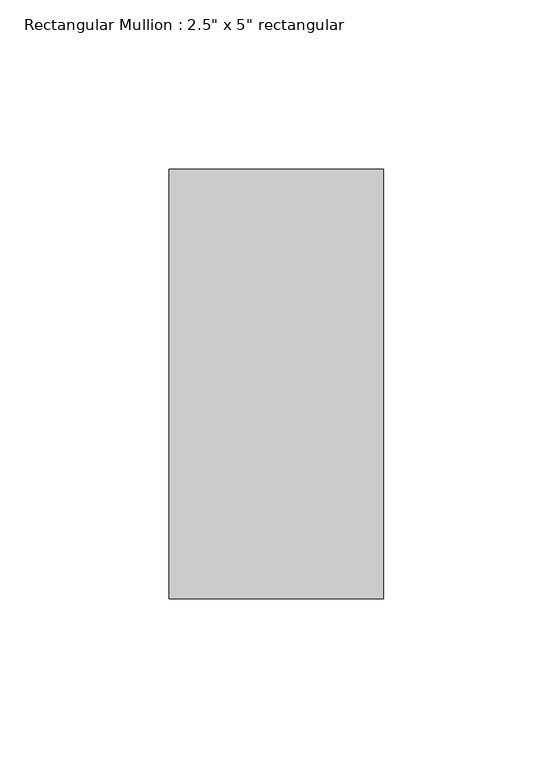
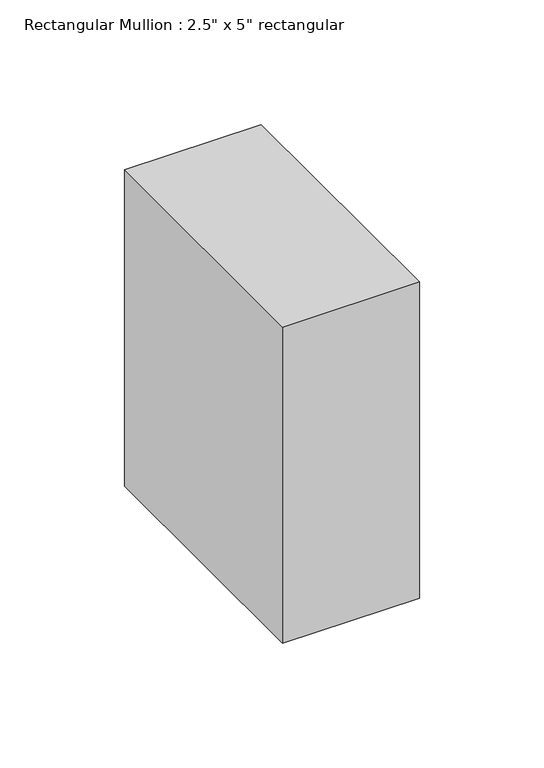
"""IFC4 building model written with IfcOpenShell, lengths in millimetres: member geometry."""

from ifc_helpers import new_model, si_unit, frame, origin, place, context, project, spatial, polyline, outline, extrude, source, transform, mapped, element, save


def member_6ed1261f(model_context):
    return source(origin(), model_context, "Body", "SweptSolid", [
        extrude(outline(polyline([(0.0, 63.5), (0.0, -63.5), (-63.5, -63.5), (-63.5, 63.5), (0.0, 63.5)])), frame((0.0, 0.0, -155.1187468), z_axis=(0.0, 0.0, 1.0), x_axis=(1.0, 0.0, 0.0)), (0.0, 0.0, 1.0), 155.1187468),
    ])


if __name__ == "__main__":
    model = new_model("IFC4")
    model_context = context("Model", 3, world=origin())
    ifc_project = project(units=[si_unit("LENGTHUNIT", "METRE", prefix="MILLI")], contexts=[model_context])
    site = spatial("IfcSite", under=ifc_project)
    building = spatial("IfcBuilding", under=site)
    placement = place(None, origin())
    member_shape = member_6ed1261f(model_context)
    element("IfcMember", 1, ObjectType="Rectangular Mullion : 2.5\" x 5\" rectangular", at=placement, inside=building, context=model_context, shape_type="MappedRepresentation", body=[
        mapped(member_shape, transform((0.0, 0.0, 0.0), x_axis=(1.0, 0.0, 0.0), y_axis=(0.0, 1.0, 0.0), z_axis=(0.0, 0.0, 1.0))),
    ])
    save(model, "model.ifc")

# Revit data of these elements
# Type "Rectangular Mullion : 2.5\" x 5\" rectangular"
#   built-in parameter 1007304 = 0.416667 (stored number, unit not read)
#   built-in parameter 1007301 = 0.104167 (stored number, unit not read)
#   built-in parameter 1007300 = 0.104167 (stored number, unit not read)
# Element 1 (IfcMember, "Rectangular Mullion : 2.5\" x 5\" rectangular")
#   Materials on its faces: "Aluminum"
# Materials
#   "Aluminum": class "Metal", colour RGB 247 247 247, transparency 0, Description = "Aluminum 6061", Cost = 0
